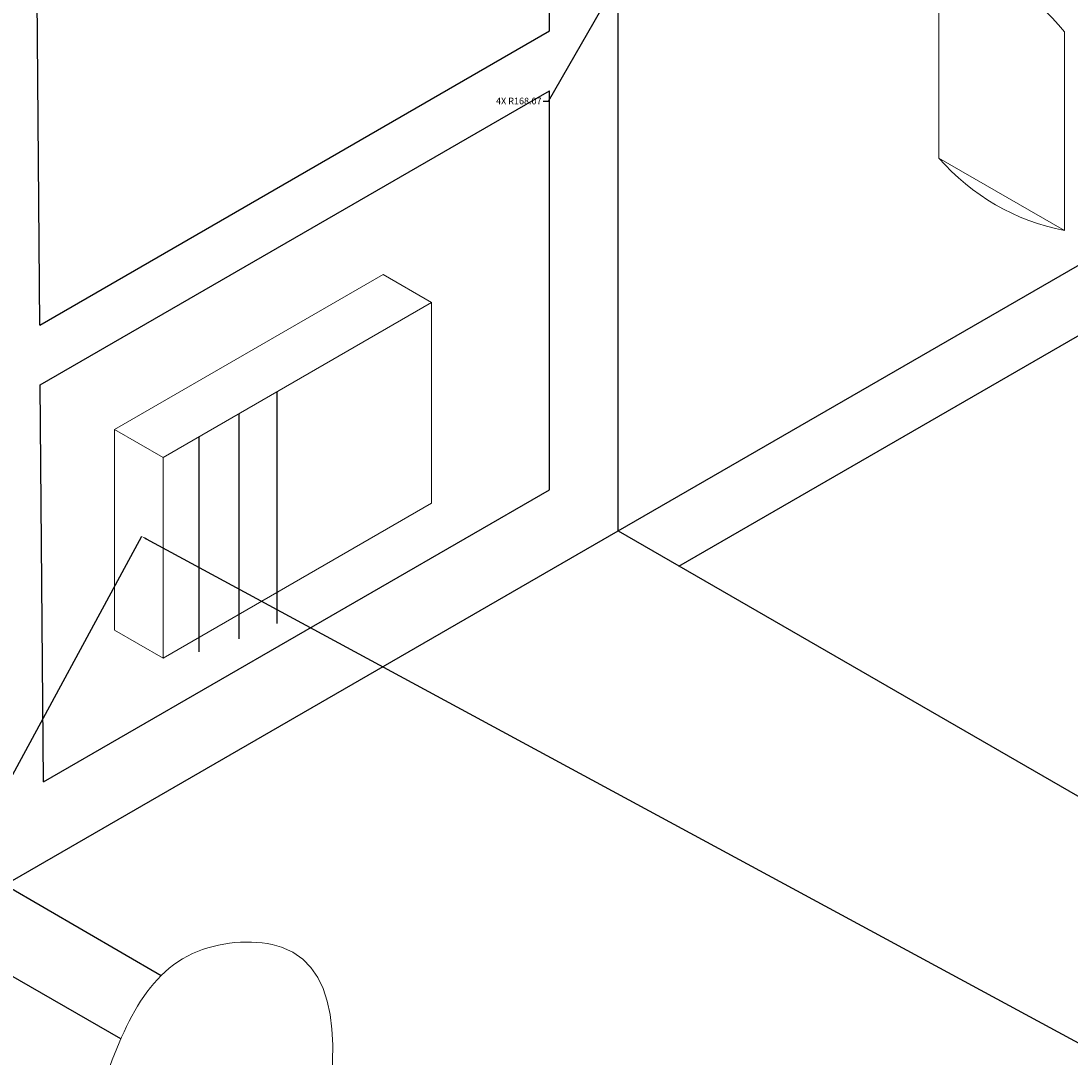
# Model space of a CAD drawing. Units: metres. Extents: x -2391 to 4922, y -635 to 4845.
# Tile 13 of 37: x -1978 to -1186, y 1408 to 2190. Entities that reach past the tile are written whole.
import ezdxf

# ---------------------------------------------------------------- set-up
doc = ezdxf.new("R2010")
doc.units = ezdxf.units.M
doc.header["$MEASUREMENT"] = 0
for name, color, linetype, lineweight in [('A-ANNO-DIMS', 2, 'Continuous', 18), ('A-EQPM', 9, 'Continuous', 18), ('A-FLOR-FIXT', 3, 'Continuous', 25), ('A-FURN', 8, 'Continuous', 18)]:
    doc.layers.add(name, color=color, linetype=linetype, lineweight=lineweight)
doc.styles.get("Standard").update_dxf_attribs({"font": 'arial.ttf'})
doc.dimstyles.get("Standard").update_dxf_attribs({"dimtxt": 5, "dimasz": 4, "dimexe": 0.18, "dimexo": 0.0625, "dimgap": 0.09, "dimtad": 0, "dimtih": 1, "dimtoh": 1, "dimdec": 0, "dimzin": 0, "dimdsep": 46, "dimtxsty": 'Standard', "dimcen": 0.09, "dimadec": 0, "dimazin": 0, "dimtfac": 1, "dimtdec": 0, "dimtofl": 0, "dimtmove": 0, "dimatfit": 3, "dimfxl": 1, "dimtolj": 1, "dimtzin": 0, "dimarcsym": 0})

# ---------------------------------------------------------------- blocks, each defined once
blk = doc.blocks.new('UTENSIL-HANGING')
for p, q in [((0, 204.54), (0, 54.7)), ((94.74, 0), (94.74, 149.84)), ((0, 54.7), (94.74, 0))]:
    blk.add_line(p, q)
for centre, radius, start, end in [((-21.43, 58.03), 148.07, 38.32024, 81.67976), ((126.83, 164.98), 168.07, 221.00715, 258.99285)]:
    blk.add_arc(centre, radius, start, end)
blk = doc.blocks.new('*D8')
at = {"layer": 'A-ANNO-DIMS', "color": 0, "lineweight": -2, "transparency": 16777216}
for p, q in [((-2047.33, 3005.21), (-2047.33, -631.4)), ((4577.76, 2350.21), (4577.76, -631.4)), ((-2043.33, -631.22), (1257.62, -631.22)), ((4573.76, -631.22), (1272.8, -631.22))]:
    blk.add_line(p, q, dxfattribs=at)
at = {"layer": 'A-ANNO-DIMS', "color": 0, "transparency": 16777216}
for points in [[(-2043.33, -630.56), (-2043.33, -631.89), (-2047.33, -631.22)], [(4573.76, -630.56), (4573.76, -631.89), (4577.76, -631.22)]]:
    blk.add_solid(points, dxfattribs=at)
at = {"layer": 'Defpoints', "color": 0, "transparency": 16777216}
for p in [(-2047.33, 3005.28), (4577.76, 2350.28), (4577.76, -631.22)]:
    blk.add_point(p, dxfattribs=at)
at = {"layer": 'A-ANNO-DIMS', "color": 0, "transparency": 16777216, "insert": (1265.21, -631.22), "char_height": 5, "attachment_point": 5}
blk.add_mtext('\\A1;6625', dxfattribs=at)
blk = doc.blocks.new('*D10')
at = {"layer": 'A-ANNO-DIMS', "color": 0, "lineweight": -2, "transparency": 16777216}
for p, q in [((550.68, 4505.28), (-2384.01, 4505.28)), ((-2383.83, 4501.28), (-2383.83, 2107.92)), ((-2383.83, -290.72), (-2383.83, 2102.63)), ((-488.55, -294.72), (-2384.01, -294.72))]:
    blk.add_line(p, q, dxfattribs=at)
at = {"layer": 'A-ANNO-DIMS', "color": 0, "transparency": 16777216}
for points in [[(-2384.5, 4501.28), (-2383.17, 4501.28), (-2383.83, 4505.28)], [(-2384.5, -290.72), (-2383.17, -290.72), (-2383.83, -294.72)]]:
    blk.add_solid(points, dxfattribs=at)
at = {"layer": 'Defpoints', "color": 0, "transparency": 16777216}
for p in [(-2383.83, 4505.28), (550.74, 4505.28), (-488.49, -294.72)]:
    blk.add_point(p, dxfattribs=at)
at = {"layer": 'A-ANNO-DIMS', "color": 0, "transparency": 16777216, "insert": (-2383.83, 2105.28), "char_height": 5, "attachment_point": 5}
blk.add_mtext('\\A1;4800', dxfattribs=at)
blk = doc.blocks.new('*D41')
at = {"layer": 'A-ANNO-DIMS', "color": 0, "lineweight": -2, "transparency": 16777216}
for p, q in [((-2047.3, 3005.33), (-1878.99, 3296.85)), ((-1875.62, 3294.69), (-1104.24, 2849.34)), ((-323.7, 2398.69), (-1095.08, 2844.05)), ((-488.46, 2105.33), (-320.15, 2396.85))]:
    blk.add_line(p, q, dxfattribs=at)
at = {"layer": 'A-ANNO-DIMS', "color": 0, "transparency": 16777216}
for points in [[(-1875.29, 3295.27), (-1875.95, 3294.12), (-1879.08, 3296.69)], [(-323.37, 2399.27), (-324.04, 2398.12), (-320.24, 2396.69)]]:
    blk.add_solid(points, dxfattribs=at)
at = {"layer": 'Defpoints', "color": 0, "transparency": 16777216}
for p in [(-2047.33, 3005.28), (-320.24, 2396.69), (-488.49, 2105.28)]:
    blk.add_point(p, dxfattribs=at)
at = {"layer": 'A-ANNO-DIMS', "color": 0, "transparency": 16777216, "insert": (-1099.66, 2846.69), "char_height": 5, "attachment_point": 5}
blk.add_mtext('\\A1;1800', dxfattribs=at)
blk = doc.blocks.new('*D46')
at = {"layer": 'A-ANNO-DIMS', "color": 0, "lineweight": -2, "transparency": 16777216}
for p, q in [((-2047.3, 1505.33), (-1887.13, 1801.4)), ((-1883.7, 1799.34), (-1087.36, 1368.5)), ((-281.24, 932.38), (-1077.58, 1363.21)), ((-437.81, 634.57), (-277.64, 930.64))]:
    blk.add_line(p, q, dxfattribs=at)
at = {"layer": 'A-ANNO-DIMS', "color": 0, "transparency": 16777216}
for points in [[(-1883.38, 1799.92), (-1884.01, 1798.75), (-1887.21, 1801.24)], [(-280.92, 932.97), (-281.56, 931.8), (-277.72, 930.48)]]:
    blk.add_solid(points, dxfattribs=at)
at = {"layer": 'Defpoints', "color": 0, "transparency": 16777216}
for p in [(-2047.33, 1505.28), (-277.72, 930.48), (-437.84, 634.52)]:
    blk.add_point(p, dxfattribs=at)
at = {"layer": 'A-ANNO-DIMS', "color": 0, "transparency": 16777216, "insert": (-1082.47, 1365.86), "char_height": 5, "attachment_point": 5}
blk.add_mtext('\\A1;1830', dxfattribs=at)
blk = doc.blocks.new('*D52')
at = {"layer": 'A-ANNO-DIMS', "color": 0, "lineweight": -2, "transparency": 16777216}
for p, q in [((-1445.98, 2362.64), (-1445.8, 2362.64)), ((-1445.89, 2362.55), (-1445.89, 2362.73)), ((-1580.35, 2129.76), (-1531.93, 2213.63)), ((-1584.35, 2129.76), (-1580.35, 2129.76))]:
    blk.add_line(p, q, dxfattribs=at)
at = {"layer": 'A-ANNO-DIMS', "color": 0, "transparency": 16777216}
blk.add_solid([(-1532.51, 2213.96), (-1531.35, 2213.29), (-1529.93, 2217.09)], dxfattribs=at)
at = {"layer": 'Defpoints', "color": 0, "transparency": 16777216}
for p in [(-1445.89, 2362.64), (-1529.93, 2217.09)]:
    blk.add_point(p, dxfattribs=at)
at = {"layer": 'A-ANNO-DIMS', "color": 0, "transparency": 16777216, "insert": (-1602.68, 2129.76), "char_height": 5, "attachment_point": 5}
blk.add_mtext('\\A1;4X R168.07', dxfattribs=at)

msp = doc.modelspace()

# ---------------------------------------------------------------- linework, layer by layer
at = {"layer": 'A-EQPM'}
for p, q in [((-1907.7708, 1881.7924), (-1705.1233, 1998.791)), ((-1668.4137, 1977.5966), (-1705.1233, 1998.791)), ((-1871.0612, 1860.5981), (-1668.4137, 1977.5966)), ((-1668.4137, 1977.5966), (-1668.4137, 1826.3302)), ((-1871.0612, 1860.5981), (-1907.7708, 1881.7924)), ((-1907.7708, 1881.7924), (-1907.7708, 1730.5259)), ((-1871.0612, 1860.5981), (-1871.0612, 1709.3316)), ((-1668.4137, 1826.3302), (-1871.0612, 1709.3316)), ((-1871.0612, 1709.3316), (-1907.7708, 1730.5259))]:
    msp.add_line(p, q, dxfattribs=at)
at = {"layer": 'A-FLOR-FIXT'}
for p, q in [((-1579.6432, 2182.6221), (-1579.6432, 2526.5253)), ((-1964.0899, 1960.6617), (-1966.7983, 2303.0012)), ((-1527.7191, 1805.2763), (-1527.7191, 2215.836)), ((-1964.0899, 1960.6617), (-1579.6432, 2182.6221)), ((-1963.7337, 1915.6336), (-1579.6432, 2137.3884)), ((-1579.6432, 1836.4354), (-1579.6432, 2137.3884)), ((-1527.7191, 1805.2763), (-968.1457, 2128.3461)), ((-1481.8951, 1778.8198), (-1013.1504, 2049.4496)), ((-1961.3635, 1616.049), (-1963.7337, 1915.6336)), ((-1785.1988, 1910.1708), (-1785.1988, 1735.5608)), ((-1813.8932, 1893.604), (-1813.8932, 1723.7996)), ((-1844.0327, 1876.203), (-1844.0327, 1713.9974)), ((-1961.3635, 1616.049), (-1579.6432, 1836.4354)), ((-2047.3343, 1505.2763), (-1527.7191, 1805.2763)), ((-1527.7191, 1805.2763), (31.1266, 905.2763)), ((-1990.2207, 1538.2508), (-1872.4955, 1469.7159)), ((-1902.9302, 1421.9045), (-2047.3343, 1505.2763))]:
    msp.add_line(p, q, dxfattribs=at)
at = {"layer": 'A-FURN'}
msp.add_open_spline([(-1526.2689, 1166.4698), (-1618.3807, 1175.9307), (-1899.5699, 1009.0778), (-1659.2657, 1504.8781), (-1879.7796, 1493.1197), (-1903.9345, 1422.9415), (-1920.3976, 1375.1107)], degree=3, knots=[588.24960444, 588.24960444, 588.24960444, 588.24960444, 753.51326986, 991.96424045, 1035.26173009, 1127.93255518, 1127.93255518, 1127.93255518, 1127.93255518], dxfattribs=at)

# ---------------------------------------------------------------- block references
at = {"layer": 'A-EQPM'}
msp.add_blockref('UTENSIL-HANGING', (-1285.7891, 2032.0011), dxfattribs=at)

# ---------------------------------------------------------------- dimensions: what is measured, and where the dimension line sits
at = {"layer": 'A-ANNO-DIMS'}
for base, p1, p2, angle, picture, middle in [((-2383.8343, 4505.2763), (-488.4886, -294.7237), (550.7419, 4505.2763), 90, '*D10', (-2383.8343, 2105.2763)), ((-320.2386, 2396.6938), (-2047.3343, 3005.2763), (-488.4886, 2105.2763), 330, '*D41', (-1099.6615, 2846.6938)), ((-277.7211, 930.4802), (-2047.3343, 1505.2763), (-437.841, 634.5176), 331.5859855, '*D46', (-1082.4677, 1365.8595))]:
    dim = msp.add_linear_dim(base=base, p1=p1, p2=p2, angle=angle, dimstyle='Standard', override={"dimdec": 0, "dimlfac": 1, "dimrnd": 0, "dimzin": 0, "dimdsep": 46, "dimlunit": 2}, dxfattribs=at)
    dim.commit()
    dim.dimension.update_dxf_attribs({"geometry": picture, "text_midpoint": middle})
dim = msp.add_linear_dim(base=(4577.76, -631.2237), p1=(-2047.3343, 3005.2763), p2=(4577.76, 2350.2763), dimstyle='Standard', override={"dimdec": 0, "dimlfac": 1, "dimrnd": 0, "dimzin": 0, "dimdsep": 46, "dimlunit": 2}, dxfattribs=at)
dim.commit()
dim.dimension.update_dxf_attribs({"geometry": '*D8', "text_midpoint": (1265.2128, -631.2237)})
dim = msp.add_radius_dim(center=(-1445.8912, 2362.6446), mpoint=(-1529.9279, 2217.0891), text='4X <>', dimstyle='Standard', override={"dimdec": 2, "dimlfac": 1, "dimrnd": 0, "dimzin": 0, "dimdsep": 46, "dimlunit": 2}, dxfattribs=at)
dim.commit()
dim.dimension.update_dxf_attribs({"geometry": '*D52', "text_midpoint": (-1602.6835, 2129.7559), "dimtype": 164})

doc.saveas('drawing.dxf')
